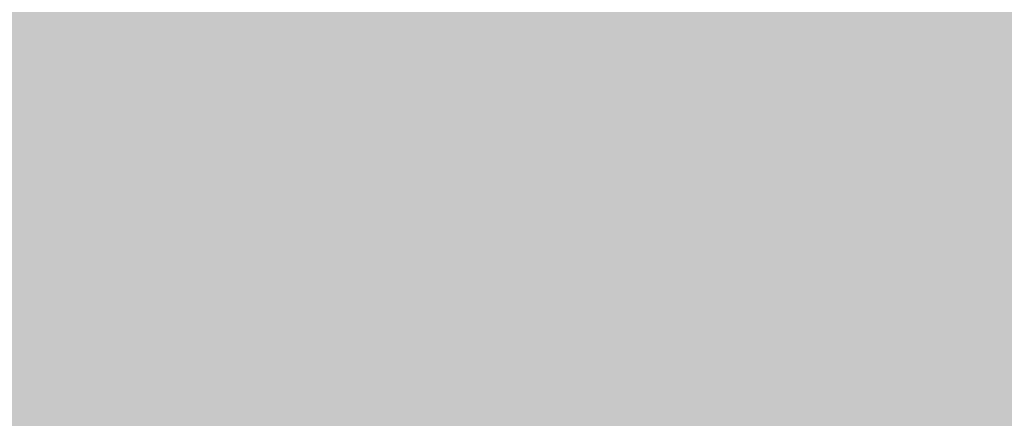
# Model space of a CAD drawing. Units: millimetres. Extents: x 0 to 2267, y 0 to 1823.
# Tile 130 of 256: x 1605.705 to 1611.042, y 1232.602 to 1234.764. Entities that reach past the tile are written whole.
import ezdxf

# ---------------------------------------------------------------- set-up
doc = ezdxf.new("R2010")
doc.units = ezdxf.units.MM
doc.header["$MEASUREMENT"] = 0
doc.layers.add('M-HATC', color=252, linetype='Continuous', lineweight=18)

msp = doc.modelspace()

# ---------------------------------------------------------------- hatches: boundary and pattern name
at = {"layer": 'M-HATC'}
h = msp.add_hatch(color=256, dxfattribs=at)
h.dxf.hatch_style = 1
h.paths.add_polyline_path([(2065.771, 1618.062, 0.236068), (2055.771, 1638.062), (1381.0868, 1638.062, 0.236068), (1371.0868, 1618.062), (1371.0868, 1603.062), (2055.771, 1603.062), (2065.771, 1603.062)])
h.paths.add_polyline_path([(2062.7718, 1550.2964), (2062.7718, 1560.2964), (1374.086, 1560.2964), (1374.086, 1550.2964), (1374.086, 1540.2964), (1384.086, 1540.2964), (1389.086, 1540.2964), (2062.7718, 1540.2964)])
h.paths.add_polyline_path([(1930.9289, 1282.7656), (1505.9289, 1282.7656), (1587.6276, 1235.5968, 0.131652), (1600.1276, 1232.2475), (1836.7302, 1232.2475, 0.131652), (1849.2302, 1235.5968)])
h.paths.add_polyline_path([(1930.9289, 1117.4171), (1905.9289, 1117.4171), (1505.9289, 1117.4171), (1505.9289, 1077.4171), (1930.9289, 1077.4171)])
h = msp.add_hatch(color=256, dxfattribs=at)
h.dxf.hatch_style = 1
h.paths.add_polyline_path([(2055.771, 1603.062), (1381.0868, 1603.062), (1381.0868, 1598.062), (2055.771, 1598.062)])
h.paths.add_polyline_path([(2055.771, 1598.062), (1381.0868, 1598.062), (1381.0868, 1593.062), (2055.771, 1593.062)])
h.paths.add_polyline_path([(2051.3074, 1536.7609), (1385.5504, 1536.7609), (1385.5504, 1526.7609), (1387.5504, 1526.7609), (1388.5366, 1525.0528), (1385.3319, 1521.2335), (1385.3319, 1521.2226), (2050.2542, 1522.7491), (2048.3212, 1525.0528), (2049.3074, 1526.7609), (2051.3074, 1526.7609)])
edge = h.paths.add_edge_path()
edge.add_arc((1847.5345, 1379.1492), 135, 222.603061, 222.890851, ccw=False)
edge.add_line((1748.1663, 1287.7656), (1683.0921, 1287.7656))
edge.add_arc((1583.7239, 1379.1492), 135, 317.109149, 317.396939, ccw=False)
edge.add_arc((1678.9686, 1290.6707), 5, 222.8909, 317.1091, ccw=False)
edge.add_arc((1774.2133, 1379.1492), 135, 222.603061, 222.890851, ccw=False)
edge.add_line((1674.8451, 1287.7656), (1609.7709, 1287.7656))
edge.add_arc((1510.4027, 1379.1492), 135, 317.109149, 317.396939, ccw=False)
edge.add_arc((1605.6474, 1290.6707), 5, 222.8909, 317.1091, ccw=False)
edge.add_arc((1700.8921, 1379.1492), 135, 222.603061, 222.890851, ccw=False)
edge.add_line((1601.5239, 1287.7656), (1536.4497, 1287.7656))
edge.add_arc((1437.0815, 1379.1492), 135, 317.109149, 317.396939, ccw=False)
edge.add_arc((1532.3262, 1290.6707), 5, 222.8909, 317.1091, ccw=False)
edge.add_arc((1627.5709, 1379.1492), 135, 222.603061, 222.890851, ccw=False)
edge.add_line((1528.2027, 1287.7656), (1505.9289, 1287.7656))
edge.add_spline(control_points=[(1505.9289, 1287.7656), (1504.2622, 1287.7656), (1504.2622, 1282.7656), (1505.9289, 1282.7656)], knot_values=[0, 0, 0, 0, 5, 5, 5, 5], degree=3, periodic=0)
edge.add_line((1505.9289, 1282.7656), (1930.9289, 1282.7656))
edge.add_spline(control_points=[(1930.9289, 1282.7656), (1932.5956, 1282.7656), (1932.5956, 1287.7656), (1930.9289, 1287.7656)], knot_values=[0, 0, 0, 0, 5, 5, 5, 5], degree=3, periodic=0)
edge.add_line((1930.9289, 1287.7656), (1903.0557, 1287.7656))
edge.add_arc((1803.6875, 1379.1492), 135, 317.109149, 317.396939, ccw=False)
edge.add_arc((1898.9322, 1290.6707), 5, 222.8909, 317.1091, ccw=False)
edge.add_arc((1994.1769, 1379.1492), 135, 222.603061, 222.890851, ccw=False)
edge.add_line((1894.8087, 1287.7656), (1829.7345, 1287.7656))
edge.add_arc((1730.3663, 1379.1492), 135, 317.109149, 317.396939, ccw=False)
edge.add_arc((1825.611, 1290.6707), 5, 222.8909, 317.1091, ccw=False)
edge.add_arc((1920.8557, 1379.1492), 135, 222.603061, 222.890851, ccw=False)
edge.add_line((1821.4875, 1287.7656), (1756.4133, 1287.7656))
edge.add_arc((1657.0451, 1379.1492), 135, 317.109149, 317.396939, ccw=False)
edge.add_arc((1752.2898, 1290.6707), 5, 222.8909, 317.1091, ccw=False)
edge = h.paths.add_edge_path()
edge.add_spline(control_points=[(1843.4289, 1227.2475), (1845.0956, 1227.2475), (1845.0956, 1232.2475), (1843.4289, 1232.2475)], knot_values=[0, 0, 0, 0, 5, 5, 5, 5], degree=3, periodic=0)
edge.add_line((1843.4289, 1232.2475), (1593.4289, 1232.2475))
edge.add_spline(control_points=[(1593.4289, 1232.2475), (1591.7622, 1232.2475), (1591.7622, 1227.2475), (1593.4289, 1227.2475)], knot_values=[0, 0, 0, 0, 5, 5, 5, 5], degree=3, periodic=0)
edge.add_line((1593.4289, 1227.2475), (1843.4289, 1227.2475))
h.paths.add_polyline_path([(1905.9289, 1127.4171), (1530.9289, 1127.4171, 0.414214), (1520.9289, 1117.4171), (1530.9289, 1117.4171), (1915.9289, 1117.4171, 0.414214)])
edge = h.paths.add_edge_path()
edge.add_arc((1397.0858, 1498.4078), 12.7299, 90.78215, 190.87871, ccw=False)
edge.add_line((1396.912, 1511.1365), (1428.0097, 1511.3488))
edge.add_line((1428.0097, 1511.3488), (1433.0097, 1511.3488))
edge.add_line((1433.0097, 1511.3488), (1434.439, 1511.3488))
edge.add_arc((1419.474, 1498.0804), 20, 41.561, 74.08211)
edge.add_line((1424.9592, 1517.3135), (1399.9351, 1517.2561))
edge.add_spline(control_points=[(1399.9307, 1517.2561), (1399.884, 1517.2131), (1399.8328, 1517.1689), (1399.7774, 1517.1236)], knot_values=[11.567499, 11.567499, 11.567499, 11.567499, 11.814249, 11.814249, 11.814249, 11.814249], degree=3, periodic=0)
edge.add_spline(control_points=[(1399.6328, 1517.0099), (1399.5831, 1516.9721), (1399.5307, 1516.9338), (1399.4759, 1516.8947)], knot_values=[11.167718, 11.167718, 11.167718, 11.167718, 11.365188, 11.365188, 11.365188, 11.365188], degree=3, periodic=0)
edge.add_spline(control_points=[(1399.3398, 1516.8001), (1399.1514, 1516.6719), (1398.9384, 1516.5377), (1398.704, 1516.3994)], knot_values=[10.376405, 10.376405, 10.376405, 10.376405, 11.00994, 11.00994, 11.00994, 11.00994], degree=3, periodic=0)
edge.add_spline(control_points=[(1398.6572, 1516.3719), (1398.5789, 1516.326), (1398.4983, 1516.2797), (1398.4155, 1516.2331)], knot_values=[10.125175, 10.125175, 10.125175, 10.125175, 10.334406, 10.334406, 10.334406, 10.334406], degree=3, periodic=0)
edge.add_spline(control_points=[(1398.2642, 1516.1487), (1398.196, 1516.1111), (1398.1263, 1516.0732), (1398.0555, 1516.0351)], knot_values=[9.832246, 9.832246, 9.832246, 9.832246, 9.999658, 9.999658, 9.999658, 9.999658], degree=3, periodic=0)
edge.add_spline(control_points=[(1397.9987, 1516.0048), (1397.7312, 1515.8621), (1397.446, 1515.7171), (1397.1466, 1515.5714)], knot_values=[9.161808, 9.161808, 9.161808, 9.161808, 9.787769, 9.787769, 9.787769, 9.787769], degree=3, periodic=0)
edge.add_spline(control_points=[(1397.1466, 1515.5714), (1396.8418, 1515.423), (1396.5222, 1515.274), (1396.1914, 1515.1262)], knot_values=[8.524455, 8.524455, 8.524455, 8.524455, 9.161808, 9.161808, 9.161808, 9.161808], degree=3, periodic=0)
edge.add_spline(control_points=[(1396.0777, 1515.0756), (1395.9854, 1515.0348), (1395.8922, 1514.994), (1395.7983, 1514.9534)], knot_values=[8.275193, 8.275193, 8.275193, 8.275193, 8.451726, 8.451726, 8.451726, 8.451726], degree=3, periodic=0)
edge.add_spline(control_points=[(1395.6018, 1514.8691), (1395.4997, 1514.8257), (1395.3968, 1514.7824), (1395.2932, 1514.7394)], knot_values=[7.962917, 7.962917, 7.962917, 7.962917, 8.152764, 8.152764, 8.152764, 8.152764], degree=3, periodic=0)
edge.add_spline(control_points=[(1395.2116, 1514.7057), (1394.8278, 1514.5475), (1394.4345, 1514.3929), (1394.0364, 1514.2442)], knot_values=[7.21254, 7.21254, 7.21254, 7.21254, 7.913148, 7.913148, 7.913148, 7.913148], degree=3, periodic=0)
edge.add_spline(control_points=[(1394.0364, 1514.2442), (1393.7076, 1514.1214), (1393.3754, 1514.0027), (1393.0427, 1513.8895)], knot_values=[6.633733, 6.633733, 6.633733, 6.633733, 7.21254, 7.21254, 7.21254, 7.21254], degree=3, periodic=0)
edge.add_spline(control_points=[(1392.8214, 1513.815), (1392.7198, 1513.7812), (1392.6181, 1513.7479), (1392.5166, 1513.7152)], knot_values=[6.328796, 6.328796, 6.328796, 6.328796, 6.505493, 6.505493, 6.505493, 6.505493], degree=3, periodic=0)
edge.add_spline(control_points=[(1392.5166, 1513.7152), (1392.3187, 1513.6515), (1392.1212, 1513.59), (1391.9244, 1513.531)], knot_values=[5.984605, 5.984605, 5.984605, 5.984605, 6.328796, 6.328796, 6.328796, 6.328796], degree=3, periodic=0)
edge.add_spline(control_points=[(1391.7915, 1513.4915), (1391.3122, 1513.3501), (1390.8384, 1513.2239), (1390.3784, 1513.1171)], knot_values=[5.066697, 5.066697, 5.066697, 5.066697, 5.907055, 5.907055, 5.907055, 5.907055], degree=3, periodic=0)
edge.add_spline(control_points=[(1390.3784, 1513.1171), (1390.1797, 1513.071), (1389.9836, 1513.0284), (1389.7907, 1512.9899)], knot_values=[4.70367, 4.70367, 4.70367, 4.70367, 5.066695, 5.066695, 5.066695, 5.066695], degree=3, periodic=0)
edge.add_spline(control_points=[(1389.422, 1512.9204), (1389.2459, 1512.8892), (1389.0729, 1512.8617), (1388.9036, 1512.8381)], knot_values=[4.130571, 4.130571, 4.130571, 4.130571, 4.469816, 4.469816, 4.469816, 4.469816], degree=3, periodic=0)
edge.add_spline(control_points=[(1388.9036, 1512.8381), (1388.591, 1512.7946), (1388.2911, 1512.7644), (1388.0071, 1512.7494)], knot_values=[3.504031, 3.504031, 3.504031, 3.504031, 4.130571, 4.130571, 4.130571, 4.130571], degree=3, periodic=0)
edge.add_spline(control_points=[(1387.9356, 1512.7459), (1387.8538, 1512.7423), (1387.7733, 1512.74), (1387.6944, 1512.739)], knot_values=[3.268866, 3.268866, 3.268866, 3.268866, 3.451164, 3.451164, 3.451164, 3.451164], degree=3, periodic=0)
edge.add_spline(control_points=[(1387.3351, 1512.7443), (1387.2076, 1512.7499), (1387.0847, 1512.7597), (1386.967, 1512.7739)], knot_values=[2.670686, 2.670686, 2.670686, 2.670686, 2.984, 2.984, 2.984, 2.984], degree=3, periodic=0)
edge.add_spline(control_points=[(1386.8327, 1512.7922), (1386.8209, 1512.7941), (1386.8092, 1512.7959), (1386.7975, 1512.7979)], knot_values=[2.516981, 2.516981, 2.516981, 2.516981, 2.549528, 2.549528, 2.549528, 2.549528], degree=3, periodic=0)
edge.add_spline(control_points=[(1386.4526, 1512.8735), (1386.4257, 1512.881), (1386.3993, 1512.889), (1386.3733, 1512.8972)], knot_values=[2.095869, 2.095869, 2.095869, 2.095869, 2.17941, 2.17941, 2.17941, 2.17941], degree=3, periodic=0)
edge.add_spline(control_points=[(1386.0691, 1513.0189), (1386.0634, 1513.0217), (1386.0577, 1513.0246), (1386.052, 1513.0275)], knot_values=[1.72453, 1.72453, 1.72453, 1.72453, 1.745933, 1.745933, 1.745933, 1.745933], degree=3, periodic=0)
edge.add_arc((1399.474, 1498.0804), 20, 131.82432, 180)
edge.add_arc((1630.3336, 1505.5484), 250.9708, 181.705176, 236.427975)
edge.add_arc((1605.3399, 1483.3044), 218.7822, 238.660829, 243.34961)
edge.add_arc((1647.0911, 1510.3592), 262.8986, 183.129836, 237.853442, ccw=False)
h.paths.add_polyline_path([(1406.5369, 1391.9644, 0.149382), (1491.5506, 1296.4418, -0.129517)], flags=17)
edge = h.paths.add_edge_path()
edge.add_arc((2037.3838, 1498.0804), 20, 0, 48.26587)
edge.add_spline(control_points=[(2050.6973, 1513.0052), (2050.6512, 1512.9847), (2050.6034, 1512.9655), (2050.5539, 1512.9477)], knot_values=[1.835652, 1.835652, 1.835652, 1.835652, 2.000781, 2.000781, 2.000781, 2.000781], degree=3, periodic=0)
edge.add_spline(control_points=[(2050.4616, 1512.9166), (2050.479, 1512.9221), (2050.4963, 1512.9277), (2050.5133, 1512.9335)], knot_values=[2.045477, 2.045477, 2.045477, 2.045477, 2.101389, 2.101389, 2.101389, 2.101389], degree=3, periodic=0)
edge.add_spline(control_points=[(2050.129, 1512.8342), (2050.1984, 1512.8473), (2050.2657, 1512.8623), (2050.3308, 1512.8792)], knot_values=[2.237629, 2.237629, 2.237629, 2.237629, 2.435841, 2.435841, 2.435841, 2.435841], degree=3, periodic=0)
edge.add_spline(control_points=[(2050.0946, 1512.8278), (2050.1061, 1512.8299), (2050.1176, 1512.832), (2050.129, 1512.8342)], knot_values=[2.435841, 2.435841, 2.435841, 2.435841, 2.468321, 2.468321, 2.468321, 2.468321], degree=3, periodic=0)
edge.add_spline(control_points=[(2049.7843, 1512.7851), (2049.8552, 1512.7922), (2049.9243, 1512.8008), (2049.9917, 1512.8109)], knot_values=[2.563852, 2.563852, 2.563852, 2.563852, 2.748541, 2.748541, 2.748541, 2.748541], degree=3, periodic=0)
edge.add_spline(control_points=[(2049.4052, 1512.7617), (2049.5364, 1512.7653), (2049.6629, 1512.773), (2049.7843, 1512.7851)], knot_values=[2.748541, 2.748541, 2.748541, 2.748541, 3.064882, 3.064882, 3.064882, 3.064882], degree=3, periodic=0)
edge.add_spline(control_points=[(2049.1698, 1512.7597), (2049.2336, 1512.7591), (2049.2965, 1512.7594), (2049.3584, 1512.7606)], knot_values=[3.102309, 3.102309, 3.102309, 3.102309, 3.2503, 3.2503, 3.2503, 3.2503], degree=3, periodic=0)
edge.add_spline(control_points=[(2048.8573, 1512.7691), (2048.9638, 1512.7638), (2049.068, 1512.7606), (2049.1698, 1512.7597)], knot_values=[3.2503, 3.2503, 3.2503, 3.2503, 3.486069, 3.486069, 3.486069, 3.486069], degree=3, periodic=0)
edge.add_spline(control_points=[(2048.6924, 1512.7789), (2048.3729, 1512.8009), (2048.0345, 1512.8411), (2047.6817, 1512.897)], knot_values=[3.606429, 3.606429, 3.606429, 3.606429, 4.2989, 4.2989, 4.2989, 4.2989], degree=3, periodic=0)
edge.add_spline(control_points=[(2047.6817, 1512.897), (2047.5458, 1512.9185), (2047.4077, 1512.9424), (2047.2678, 1512.9685)], knot_values=[4.2989, 4.2989, 4.2989, 4.2989, 4.565769, 4.565769, 4.565769, 4.565769], degree=3, periodic=0)
edge.add_spline(control_points=[(2047.2678, 1512.9685), (2047.1449, 1512.9914), (2047.0207, 1513.016), (2046.8951, 1513.0422)], knot_values=[4.565769, 4.565769, 4.565769, 4.565769, 4.799971, 4.799971, 4.799971, 4.799971], degree=3, periodic=0)
edge.add_spline(control_points=[(2046.8951, 1513.0422), (2046.5286, 1513.1188), (2046.1513, 1513.209), (2045.7676, 1513.3107)], knot_values=[4.799971, 4.799971, 4.799971, 4.799971, 5.483718, 5.483718, 5.483718, 5.483718], degree=3, periodic=0)
edge.add_spline(control_points=[(2045.7676, 1513.3107), (2045.3724, 1513.4154), (2044.9704, 1513.5322), (2044.5662, 1513.6588)], knot_values=[5.483718, 5.483718, 5.483718, 5.483718, 6.187866, 6.187866, 6.187866, 6.187866], degree=3, periodic=0)
edge.add_spline(control_points=[(2044.5662, 1513.6588), (2044.4149, 1513.7061), (2044.2633, 1513.7549), (2044.1116, 1513.8048)], knot_values=[6.187866, 6.187866, 6.187866, 6.187866, 6.451551, 6.451551, 6.451551, 6.451551], degree=3, periodic=0)
edge.add_spline(control_points=[(2044.1116, 1513.8048), (2043.9967, 1513.8427), (2043.8817, 1513.8813), (2043.7668, 1513.9205)], knot_values=[6.451551, 6.451551, 6.451551, 6.451551, 6.651434, 6.651434, 6.651434, 6.651434], degree=3, periodic=0)
edge.add_spline(control_points=[(2043.7668, 1513.9205), (2043.3716, 1514.0554), (2042.9774, 1514.1979), (2042.5886, 1514.3458)], knot_values=[6.651434, 6.651434, 6.651434, 6.651434, 7.338879, 7.338879, 7.338879, 7.338879], degree=3, periodic=0)
edge.add_spline(control_points=[(2042.5886, 1514.3458), (2042.1643, 1514.5071), (2041.7465, 1514.6749), (2041.3409, 1514.846)], knot_values=[7.338879, 7.338879, 7.338879, 7.338879, 8.089209, 8.089209, 8.089209, 8.089209], degree=3, periodic=0)
edge.add_spline(control_points=[(2041.3409, 1514.846), (2041.1028, 1514.9465), (2040.869, 1515.0481), (2040.6405, 1515.1502)], knot_values=[8.089209, 8.089209, 8.089209, 8.089209, 8.529587, 8.529587, 8.529587, 8.529587], degree=3, periodic=0)
edge.add_spline(control_points=[(2040.51, 1515.2089), (2040.0824, 1515.4022), (2039.6747, 1515.5971), (2039.295, 1515.7894)], knot_values=[8.613818, 8.613818, 8.613818, 8.613818, 9.44571, 9.44571, 9.44571, 9.44571], degree=3, periodic=0)
edge.add_spline(control_points=[(2039.295, 1515.7894), (2039.0618, 1515.9075), (2038.8391, 1516.0246), (2038.6288, 1516.1398)], knot_values=[9.44571, 9.44571, 9.44571, 9.44571, 9.956404, 9.956404, 9.956404, 9.956404], degree=3, periodic=0)
edge.add_spline(control_points=[(2038.6288, 1516.1398), (2038.5187, 1516.2001), (2038.4121, 1516.2598), (2038.309, 1516.3189)], knot_values=[9.956404, 9.956404, 9.956404, 9.956404, 10.223542, 10.223542, 10.223542, 10.223542], degree=3, periodic=0)
edge.add_spline(control_points=[(2038.309, 1516.3189), (2038.2138, 1516.3735), (2038.1216, 1516.4276), (2038.0328, 1516.481)], knot_values=[10.223542, 10.223542, 10.223542, 10.223542, 10.47051, 10.47051, 10.47051, 10.47051], degree=3, periodic=0)
edge.add_spline(control_points=[(2038.0328, 1516.481), (2037.7855, 1516.6296), (2037.5639, 1516.773), (2037.3722, 1516.909)], knot_values=[10.47051, 10.47051, 10.47051, 10.47051, 11.15767, 11.15767, 11.15767, 11.15767], degree=3, periodic=0)
edge.add_spline(control_points=[(2037.3722, 1516.909), (2037.2789, 1516.9752), (2037.1927, 1517.0396), (2037.1142, 1517.102)], knot_values=[11.15767, 11.15767, 11.15767, 11.15767, 11.49227, 11.49227, 11.49227, 11.49227], degree=3, periodic=0)
edge.add_spline(control_points=[(2036.8564, 1517.3259), (2036.9148, 1517.2692), (2036.9814, 1517.2103), (2037.0557, 1517.1492)], knot_values=[11.577341, 11.577341, 11.577341, 11.577341, 11.91035, 11.91035, 11.91035, 11.91035], degree=3, periodic=0)
edge.add_spline(control_points=[(2036.8074, 1517.3748), (2036.823, 1517.3587), (2036.8393, 1517.3424), (2036.8564, 1517.3259)], knot_values=[11.91035, 11.91035, 11.91035, 11.91035, 12.007402, 12.007402, 12.007402, 12.007402], degree=3, periodic=0)
edge.add_spline(control_points=[(2036.7017, 1517.494), (2036.7104, 1517.483), (2036.7196, 1517.4719), (2036.7291, 1517.4606)], knot_values=[12.184155, 12.184155, 12.184155, 12.184155, 12.255409, 12.255409, 12.255409, 12.255409], degree=3, periodic=0)
edge.add_spline(control_points=[(2036.6159, 1517.6205), (2036.62, 1517.613), (2036.6243, 1517.6055), (2036.6289, 1517.5979)], knot_values=[12.487913, 12.487913, 12.487913, 12.487913, 12.541035, 12.541035, 12.541035, 12.541035], degree=3, periodic=0)
edge.add_spline(control_points=[(2036.5635, 1517.786), (2036.5637, 1517.7794), (2036.5642, 1517.7726), (2036.565, 1517.7658)], knot_values=[12.911761, 12.911761, 12.911761, 12.911761, 12.968286, 12.968286, 12.968286, 12.968286], degree=3, periodic=0)
edge.add_spline(control_points=[(2036.6166, 1517.9304), (2036.6125, 1517.9259), (2036.6086, 1517.9212), (2036.6049, 1517.9165)], knot_values=[13.382527, 13.382527, 13.382527, 13.382527, 13.433791, 13.433791, 13.433791, 13.433791], degree=3, periodic=0)
edge.add_spline(control_points=[(2036.749, 1518.017), (2036.7361, 1518.0116), (2036.7239, 1518.006), (2036.7124, 1518.0002)], knot_values=[13.726299, 13.726299, 13.726299, 13.726299, 13.809928, 13.809928, 13.809928, 13.809928], degree=3, periodic=0)
edge.add_spline(control_points=[(2036.8604, 1518.0528), (2036.8386, 1518.0474), (2036.8181, 1518.0416), (2036.7988, 1518.0353)], knot_values=[13.910887, 13.910887, 13.910887, 13.910887, 14.02153, 14.02153, 14.02153, 14.02153], degree=3, periodic=0)
edge.add_line((2036.9639, 1518.0804), (2032.3838, 1518.0804))
edge.add_line((2032.3838, 1518.0804), (2027.3838, 1518.0804))
edge.add_line((2027.3838, 1518.0804), (2022.3838, 1518.0804))
edge.add_line((2022.3838, 1518.0804), (2017.3838, 1518.0804))
edge.add_arc((2017.3838, 1498.0804), 20, 90, 138.439)
edge.add_line((2002.4188, 1511.3488), (2003.8481, 1511.3488))
edge.add_line((2003.8481, 1511.3488), (2008.8481, 1511.3488))
edge.add_line((2008.8481, 1511.3488), (2039.772, 1511.1377))
edge.add_arc((2039.772, 1498.4078), 12.7299, -10.87871, 90, ccw=False)
edge.add_arc((1789.7668, 1510.3592), 262.8986, 302.146558, 356.870164, ccw=False)
edge.add_arc((1831.5179, 1483.3044), 218.7822, 296.65039, 301.339171)
edge.add_arc((1806.5242, 1505.5484), 250.9708, 303.572025, 358.294824)
h.paths.add_polyline_path([(2030.321, 1391.9644, -0.129517), (1945.3072, 1296.4418, 0.149382)], flags=17)
edge = h.paths.add_edge_path()
edge.add_spline(control_points=[(2037.2464, 1518.0821), (2037.2898, 1518.081), (2037.3355, 1518.0804), (2037.3838, 1518.0804)], knot_values=[0.000012, 0.000012, 0.000012, 0.000012, 0.144754, 0.144754, 0.144754, 0.144754], degree=3, periodic=0)
edge.add_line((2037.3357, 1518.0804), (2037.0096, 1518.0804))
edge.add_spline(control_points=[(2037.0096, 1518.0804), (2036.9822, 1518.0768), (2036.956, 1518.0727), (2036.9312, 1518.0681)], knot_values=[14.13465, 14.13465, 14.13465, 14.13465, 14.247197, 14.247197, 14.247197, 14.247197], degree=3, periodic=0)
edge.add_spline(control_points=[(2036.9312, 1518.0681), (2036.9276, 1518.0674), (2036.9241, 1518.0667), (2036.9205, 1518.0661)], knot_values=[14.118315, 14.118315, 14.118315, 14.118315, 14.13465, 14.13465, 14.13465, 14.13465], degree=3, periodic=0)
edge.add_spline(control_points=[(2036.9205, 1518.0661), (2036.9118, 1518.0644), (2036.9032, 1518.0626), (2036.8948, 1518.0608)], knot_values=[14.078086, 14.078086, 14.078086, 14.078086, 14.118315, 14.118315, 14.118315, 14.118315], degree=3, periodic=0)
edge.add_spline(control_points=[(2036.8948, 1518.0608), (2036.883, 1518.0583), (2036.8716, 1518.0556), (2036.8604, 1518.0528)], knot_values=[14.02153, 14.02153, 14.02153, 14.02153, 14.078086, 14.078086, 14.078086, 14.078086], degree=3, periodic=0)
edge.add_spline(control_points=[(2036.8604, 1518.0528), (2036.8386, 1518.0474), (2036.8181, 1518.0416), (2036.7988, 1518.0353)], knot_values=[13.910887, 13.910887, 13.910887, 13.910887, 14.02153, 14.02153, 14.02153, 14.02153], degree=3, periodic=0)
edge.add_spline(control_points=[(2036.7988, 1518.0353), (2036.7981, 1518.035), (2036.7974, 1518.0348), (2036.7967, 1518.0346)], knot_values=[13.906906, 13.906906, 13.906906, 13.906906, 13.910887, 13.910887, 13.910887, 13.910887], degree=3, periodic=0)
edge.add_spline(control_points=[(2036.7967, 1518.0346), (2036.7882, 1518.0318), (2036.7799, 1518.0289), (2036.7719, 1518.0259)], knot_values=[13.857826, 13.857826, 13.857826, 13.857826, 13.906906, 13.906906, 13.906906, 13.906906], degree=3, periodic=0)
edge.add_spline(control_points=[(2036.7719, 1518.0259), (2036.764, 1518.023), (2036.7564, 1518.02), (2036.749, 1518.017)], knot_values=[13.809928, 13.809928, 13.809928, 13.809928, 13.857826, 13.857826, 13.857826, 13.857826], degree=3, periodic=0)
edge.add_spline(control_points=[(2036.749, 1518.017), (2036.7361, 1518.0116), (2036.7239, 1518.006), (2036.7124, 1518.0002)], knot_values=[13.726299, 13.726299, 13.726299, 13.726299, 13.809928, 13.809928, 13.809928, 13.809928], degree=3, periodic=0)
edge.add_spline(control_points=[(2036.7124, 1518.0002), (2036.7121, 1518), (2036.7118, 1517.9999), (2036.7115, 1517.9997)], knot_values=[13.723993, 13.723993, 13.723993, 13.723993, 13.726299, 13.726299, 13.726299, 13.726299], degree=3, periodic=0)
edge.add_spline(control_points=[(2036.7115, 1517.9997), (2036.7063, 1517.9971), (2036.7013, 1517.9944), (2036.6965, 1517.9917)], knot_values=[13.686536, 13.686536, 13.686536, 13.686536, 13.723993, 13.723993, 13.723993, 13.723993], degree=3, periodic=0)
edge.add_spline(control_points=[(2036.6965, 1517.9917), (2036.6919, 1517.9891), (2036.6874, 1517.9865), (2036.6831, 1517.9839)], knot_values=[13.651251, 13.651251, 13.651251, 13.651251, 13.686536, 13.686536, 13.686536, 13.686536], degree=3, periodic=0)
edge.add_spline(control_points=[(2036.6831, 1517.9839), (2036.6764, 1517.9798), (2036.67, 1517.9757), (2036.6639, 1517.9714)], knot_values=[13.596804, 13.596804, 13.596804, 13.596804, 13.651251, 13.651251, 13.651251, 13.651251], degree=3, periodic=0)
edge.add_spline(control_points=[(2036.6639, 1517.9714), (2036.6636, 1517.9712), (2036.6633, 1517.9709), (2036.6629, 1517.9707)], knot_values=[13.593956, 13.593956, 13.593956, 13.593956, 13.596804, 13.596804, 13.596804, 13.596804], degree=3, periodic=0)
edge.add_spline(control_points=[(2036.6629, 1517.9707), (2036.6603, 1517.9689), (2036.6577, 1517.967), (2036.6552, 1517.9651)], knot_values=[13.570322, 13.570322, 13.570322, 13.570322, 13.593956, 13.593956, 13.593956, 13.593956], degree=3, periodic=0)
edge.add_spline(control_points=[(2036.6552, 1517.9651), (2036.6525, 1517.9631), (2036.6499, 1517.9611), (2036.6474, 1517.9591)], knot_values=[13.545477, 13.545477, 13.545477, 13.545477, 13.570322, 13.570322, 13.570322, 13.570322], degree=3, periodic=0)
edge.add_spline(control_points=[(2036.6474, 1517.9591), (2036.6472, 1517.9589), (2036.6471, 1517.9588), (2036.6469, 1517.9587)], knot_values=[13.543931, 13.543931, 13.543931, 13.543931, 13.545477, 13.545477, 13.545477, 13.545477], degree=3, periodic=0)
edge.add_spline(control_points=[(2036.6469, 1517.9587), (2036.6412, 1517.9541), (2036.6358, 1517.9494), (2036.6307, 1517.9447)], knot_values=[13.488237, 13.488237, 13.488237, 13.488237, 13.543931, 13.543931, 13.543931, 13.543931], degree=3, periodic=0)
edge.add_spline(control_points=[(2036.6307, 1517.9447), (2036.6282, 1517.9423), (2036.6257, 1517.9399), (2036.6233, 1517.9374)], knot_values=[13.460307, 13.460307, 13.460307, 13.460307, 13.488237, 13.488237, 13.488237, 13.488237], degree=3, periodic=0)
edge.add_spline(control_points=[(2036.6233, 1517.9374), (2036.6215, 1517.9356), (2036.6198, 1517.9338), (2036.6181, 1517.932)], knot_values=[13.439712, 13.439712, 13.439712, 13.439712, 13.460307, 13.460307, 13.460307, 13.460307], degree=3, periodic=0)
edge.add_spline(control_points=[(2036.6181, 1517.932), (2036.6176, 1517.9315), (2036.6171, 1517.9309), (2036.6166, 1517.9304)], knot_values=[13.433791, 13.433791, 13.433791, 13.433791, 13.439712, 13.439712, 13.439712, 13.439712], degree=3, periodic=0)
edge.add_spline(control_points=[(2036.6166, 1517.9304), (2036.6125, 1517.9259), (2036.6086, 1517.9212), (2036.6049, 1517.9165)], knot_values=[13.382527, 13.382527, 13.382527, 13.382527, 13.433791, 13.433791, 13.433791, 13.433791], degree=3, periodic=0)
edge.add_spline(control_points=[(2036.6049, 1517.9165), (2036.6026, 1517.9135), (2036.6004, 1517.9104), (2036.5982, 1517.9074)], knot_values=[13.350017, 13.350017, 13.350017, 13.350017, 13.382527, 13.382527, 13.382527, 13.382527], degree=3, periodic=0)
edge.add_spline(control_points=[(2036.5982, 1517.9074), (2036.5972, 1517.9059), (2036.5962, 1517.9043), (2036.5952, 1517.9028)], knot_values=[13.333922, 13.333922, 13.333922, 13.333922, 13.350017, 13.350017, 13.350017, 13.350017], degree=3, periodic=0)
edge.add_spline(control_points=[(2036.5952, 1517.9028), (2036.5945, 1517.9018), (2036.5939, 1517.9009), (2036.5933, 1517.8999)], knot_values=[13.323828, 13.323828, 13.323828, 13.323828, 13.333922, 13.333922, 13.333922, 13.333922], degree=3, periodic=0)
edge.add_spline(control_points=[(2036.5933, 1517.8999), (2036.5905, 1517.8955), (2036.5879, 1517.8909), (2036.5855, 1517.8864)], knot_values=[13.277545, 13.277545, 13.277545, 13.277545, 13.323828, 13.323828, 13.323828, 13.323828], degree=3, periodic=0)
edge.add_spline(control_points=[(2036.5855, 1517.8864), (2036.5836, 1517.8827), (2036.5817, 1517.8789), (2036.5801, 1517.8751)], knot_values=[13.240119, 13.240119, 13.240119, 13.240119, 13.277545, 13.277545, 13.277545, 13.277545], degree=3, periodic=0)
edge.add_spline(control_points=[(2036.5801, 1517.8751), (2036.5795, 1517.8739), (2036.579, 1517.8727), (2036.5785, 1517.8715)], knot_values=[13.228211, 13.228211, 13.228211, 13.228211, 13.240119, 13.240119, 13.240119, 13.240119], degree=3, periodic=0)
edge.add_spline(control_points=[(2036.5785, 1517.8715), (2036.578, 1517.8702), (2036.5774, 1517.869), (2036.5769, 1517.8677)], knot_values=[13.215717, 13.215717, 13.215717, 13.215717, 13.228211, 13.228211, 13.228211, 13.228211], degree=3, periodic=0)
edge.add_spline(control_points=[(2036.5769, 1517.8677), (2036.5755, 1517.864), (2036.5741, 1517.8603), (2036.5729, 1517.8565)], knot_values=[13.179847, 13.179847, 13.179847, 13.179847, 13.215717, 13.215717, 13.215717, 13.215717], degree=3, periodic=0)
edge.add_spline(control_points=[(2036.5729, 1517.8565), (2036.5713, 1517.8515), (2036.5699, 1517.8464), (2036.5687, 1517.8413)], knot_values=[13.132017, 13.132017, 13.132017, 13.132017, 13.179847, 13.179847, 13.179847, 13.179847], degree=3, periodic=0)
edge.add_spline(control_points=[(2036.5687, 1517.8413), (2036.5684, 1517.8402), (2036.5682, 1517.8392), (2036.568, 1517.8382)], knot_values=[13.122482, 13.122482, 13.122482, 13.122482, 13.132017, 13.132017, 13.132017, 13.132017], degree=3, periodic=0)
edge.add_spline(control_points=[(2036.568, 1517.8382), (2036.5676, 1517.8363), (2036.5672, 1517.8345), (2036.5669, 1517.8327)], knot_values=[13.105592, 13.105592, 13.105592, 13.105592, 13.122482, 13.122482, 13.122482, 13.122482], degree=3, periodic=0)
edge.add_spline(control_points=[(2036.5669, 1517.8327), (2036.5662, 1517.8292), (2036.5657, 1517.8257), (2036.5652, 1517.8222)], knot_values=[13.074063, 13.074063, 13.074063, 13.074063, 13.105592, 13.105592, 13.105592, 13.105592], degree=3, periodic=0)
edge.add_spline(control_points=[(2036.5652, 1517.8222), (2036.5652, 1517.8222), (2036.5652, 1517.8222), (2036.5652, 1517.8222)], knot_values=[13.074043, 13.074043, 13.074043, 13.074043, 13.074063, 13.074063, 13.074063, 13.074063], degree=3, periodic=0)
edge.add_spline(control_points=[(2036.5652, 1517.8222), (2036.5644, 1517.8164), (2036.5639, 1517.8106), (2036.5636, 1517.8046)], knot_values=[13.021884, 13.021884, 13.021884, 13.021884, 13.074043, 13.074043, 13.074043, 13.074043], degree=3, periodic=0)
edge.add_spline(control_points=[(2036.5636, 1517.8046), (2036.5636, 1517.804), (2036.5636, 1517.8034), (2036.5635, 1517.8028)], knot_values=[13.01674, 13.01674, 13.01674, 13.01674, 13.021884, 13.021884, 13.021884, 13.021884], degree=3, periodic=0)
edge.add_spline(control_points=[(2036.5635, 1517.8028), (2036.5634, 1517.8005), (2036.5634, 1517.7982), (2036.5634, 1517.7958)], knot_values=[12.996438, 12.996438, 12.996438, 12.996438, 13.01674, 13.01674, 13.01674, 13.01674], degree=3, periodic=0)
edge.add_spline(control_points=[(2036.5634, 1517.7958), (2036.5633, 1517.7926), (2036.5634, 1517.7893), (2036.5635, 1517.786)], knot_values=[12.968286, 12.968286, 12.968286, 12.968286, 12.996438, 12.996438, 12.996438, 12.996438], degree=3, periodic=0)
edge.add_spline(control_points=[(2036.5635, 1517.786), (2036.5637, 1517.7794), (2036.5642, 1517.7726), (2036.565, 1517.7658)], knot_values=[12.911761, 12.911761, 12.911761, 12.911761, 12.968286, 12.968286, 12.968286, 12.968286], degree=3, periodic=0)
edge.add_spline(control_points=[(2036.565, 1517.7658), (2036.565, 1517.7657), (2036.565, 1517.7656), (2036.565, 1517.7656)], knot_values=[12.911017, 12.911017, 12.911017, 12.911017, 12.911761, 12.911761, 12.911761, 12.911761], degree=3, periodic=0)
edge.add_spline(control_points=[(2036.565, 1517.7656), (2036.5654, 1517.7625), (2036.5658, 1517.7593), (2036.5663, 1517.7562)], knot_values=[12.88528, 12.88528, 12.88528, 12.88528, 12.911017, 12.911017, 12.911017, 12.911017], degree=3, periodic=0)
edge.add_spline(control_points=[(2036.5663, 1517.7562), (2036.5667, 1517.7534), (2036.5672, 1517.7506), (2036.5677, 1517.7478)], knot_values=[12.862519, 12.862519, 12.862519, 12.862519, 12.88528, 12.88528, 12.88528, 12.88528], degree=3, periodic=0)
edge.add_spline(control_points=[(2036.5677, 1517.7478), (2036.5678, 1517.7474), (2036.5679, 1517.7469), (2036.568, 1517.7465)], knot_values=[12.858885, 12.858885, 12.858885, 12.858885, 12.862519, 12.862519, 12.862519, 12.862519], degree=3, periodic=0)
edge.add_spline(control_points=[(2036.568, 1517.7465), (2036.5692, 1517.7399), (2036.5707, 1517.7332), (2036.5724, 1517.7264)], knot_values=[12.8053, 12.8053, 12.8053, 12.8053, 12.858885, 12.858885, 12.858885, 12.858885], degree=3, periodic=0)
edge.add_spline(control_points=[(2036.5724, 1517.7264), (2036.5734, 1517.7226), (2036.5745, 1517.7187), (2036.5756, 1517.7149)], knot_values=[12.775176, 12.775176, 12.775176, 12.775176, 12.8053, 12.8053, 12.8053, 12.8053], degree=3, periodic=0)
edge.add_spline(control_points=[(2036.5756, 1517.7149), (2036.5763, 1517.7125), (2036.577, 1517.7102), (2036.5778, 1517.7078)], knot_values=[12.756759, 12.756759, 12.756759, 12.756759, 12.775176, 12.775176, 12.775176, 12.775176], degree=3, periodic=0)
edge.add_spline(control_points=[(2036.5778, 1517.7078), (2036.5781, 1517.7067), (2036.5784, 1517.7057), (2036.5787, 1517.7047)], knot_values=[12.748742, 12.748742, 12.748742, 12.748742, 12.756759, 12.756759, 12.756759, 12.756759], degree=3, periodic=0)
edge.add_spline(control_points=[(2036.5787, 1517.7047), (2036.5808, 1517.6983), (2036.5831, 1517.6919), (2036.5856, 1517.6854)], knot_values=[12.69959, 12.69959, 12.69959, 12.69959, 12.748742, 12.748742, 12.748742, 12.748742], degree=3, periodic=0)
edge.add_spline(control_points=[(2036.5856, 1517.6854), (2036.5876, 1517.68), (2036.5898, 1517.6746), (2036.5921, 1517.6692)], knot_values=[12.659038, 12.659038, 12.659038, 12.659038, 12.69959, 12.69959, 12.69959, 12.69959], degree=3, periodic=0)
edge.add_spline(control_points=[(2036.5921, 1517.6692), (2036.594, 1517.6648), (2036.5959, 1517.6605), (2036.5979, 1517.6561)], knot_values=[12.626806, 12.626806, 12.626806, 12.626806, 12.659038, 12.659038, 12.659038, 12.659038], degree=3, periodic=0)
edge.add_spline(control_points=[(2036.5979, 1517.6561), (2036.5984, 1517.6551), (2036.5989, 1517.6541), (2036.5993, 1517.6531)], knot_values=[12.619394, 12.619394, 12.619394, 12.619394, 12.626806, 12.626806, 12.626806, 12.626806], degree=3, periodic=0)
edge.add_spline(control_points=[(2036.5993, 1517.6531), (2036.6043, 1517.6424), (2036.6099, 1517.6315), (2036.6159, 1517.6205)], knot_values=[12.541039, 12.541039, 12.541039, 12.541039, 12.619394, 12.619394, 12.619394, 12.619394], degree=3, periodic=0)
edge.add_spline(control_points=[(2036.6159, 1517.6205), (2036.6159, 1517.6205), (2036.6159, 1517.6205), (2036.6159, 1517.6205)], knot_values=[12.541035, 12.541035, 12.541035, 12.541035, 12.541039, 12.541039, 12.541039, 12.541039], degree=3, periodic=0)
edge.add_spline(control_points=[(2036.6159, 1517.6205), (2036.62, 1517.613), (2036.6243, 1517.6055), (2036.6289, 1517.5979)], knot_values=[12.487913, 12.487913, 12.487913, 12.487913, 12.541035, 12.541035, 12.541035, 12.541035], degree=3, periodic=0)
edge.add_spline(control_points=[(2036.6289, 1517.5979), (2036.6326, 1517.5916), (2036.6365, 1517.5853), (2036.6406, 1517.5789)], knot_values=[12.443982, 12.443982, 12.443982, 12.443982, 12.487913, 12.487913, 12.487913, 12.487913], degree=3, periodic=0)
edge.add_spline(control_points=[(2036.6406, 1517.5789), (2036.6414, 1517.5776), (2036.6423, 1517.5763), (2036.6431, 1517.5749)], knot_values=[12.434996, 12.434996, 12.434996, 12.434996, 12.443982, 12.443982, 12.443982, 12.443982], degree=3, periodic=0)
edge.add_spline(control_points=[(2036.6431, 1517.5749), (2036.6531, 1517.5596), (2036.6639, 1517.5439), (2036.6756, 1517.528)], knot_values=[12.329647, 12.329647, 12.329647, 12.329647, 12.434996, 12.434996, 12.434996, 12.434996], degree=3, periodic=0)
edge.add_spline(control_points=[(2036.6756, 1517.528), (2036.6839, 1517.5168), (2036.6925, 1517.5055), (2036.7017, 1517.494)], knot_values=[12.255409, 12.255409, 12.255409, 12.255409, 12.329647, 12.329647, 12.329647, 12.329647], degree=3, periodic=0)
edge.add_spline(control_points=[(2036.7017, 1517.494), (2036.7104, 1517.483), (2036.7196, 1517.4719), (2036.7291, 1517.4606)], knot_values=[12.184155, 12.184155, 12.184155, 12.184155, 12.255409, 12.255409, 12.255409, 12.255409], degree=3, periodic=0)
edge.add_spline(control_points=[(2036.7291, 1517.4606), (2036.7436, 1517.4435), (2036.759, 1517.4262), (2036.7753, 1517.4085)], knot_values=[12.075961, 12.075961, 12.075961, 12.075961, 12.184155, 12.184155, 12.184155, 12.184155], degree=3, periodic=0)
edge.add_spline(control_points=[(2036.7753, 1517.4085), (2036.7763, 1517.4075), (2036.7773, 1517.4064), (2036.7783, 1517.4054)], knot_values=[12.069502, 12.069502, 12.069502, 12.069502, 12.075961, 12.075961, 12.075961, 12.075961], degree=3, periodic=0)
edge.add_spline(control_points=[(2036.7783, 1517.4054), (2036.7877, 1517.3953), (2036.7974, 1517.385), (2036.8074, 1517.3748)], knot_values=[12.007402, 12.007402, 12.007402, 12.007402, 12.069502, 12.069502, 12.069502, 12.069502], degree=3, periodic=0)
edge.add_spline(control_points=[(2036.8074, 1517.3748), (2036.823, 1517.3587), (2036.8393, 1517.3424), (2036.8564, 1517.3259)], knot_values=[11.91035, 11.91035, 11.91035, 11.91035, 12.007402, 12.007402, 12.007402, 12.007402], degree=3, periodic=0)
edge.add_spline(control_points=[(2036.8564, 1517.3259), (2036.9148, 1517.2692), (2036.9814, 1517.2103), (2037.0557, 1517.1492)], knot_values=[11.577341, 11.577341, 11.577341, 11.577341, 11.91035, 11.91035, 11.91035, 11.91035], degree=3, periodic=0)
edge.add_spline(control_points=[(2037.0557, 1517.1492), (2037.0747, 1517.1336), (2037.0942, 1517.1179), (2037.1142, 1517.102)], knot_values=[11.49227, 11.49227, 11.49227, 11.49227, 11.577341, 11.577341, 11.577341, 11.577341], degree=3, periodic=0)
edge.add_spline(control_points=[(2037.1142, 1517.102), (2037.1927, 1517.0396), (2037.2789, 1516.9752), (2037.3722, 1516.909)], knot_values=[11.15767, 11.15767, 11.15767, 11.15767, 11.49227, 11.49227, 11.49227, 11.49227], degree=3, periodic=0)
edge.add_spline(control_points=[(2037.3722, 1516.909), (2037.5639, 1516.773), (2037.7855, 1516.6296), (2038.0328, 1516.481)], knot_values=[10.47051, 10.47051, 10.47051, 10.47051, 11.15767, 11.15767, 11.15767, 11.15767], degree=3, periodic=0)
edge.add_spline(control_points=[(2038.0328, 1516.481), (2038.1216, 1516.4276), (2038.2138, 1516.3735), (2038.309, 1516.3189)], knot_values=[10.223542, 10.223542, 10.223542, 10.223542, 10.47051, 10.47051, 10.47051, 10.47051], degree=3, periodic=0)
edge.add_spline(control_points=[(2038.309, 1516.3189), (2038.4121, 1516.2598), (2038.5187, 1516.2001), (2038.6288, 1516.1398)], knot_values=[9.956404, 9.956404, 9.956404, 9.956404, 10.223542, 10.223542, 10.223542, 10.223542], degree=3, periodic=0)
edge.add_spline(control_points=[(2038.6288, 1516.1398), (2038.8391, 1516.0246), (2039.0618, 1515.9075), (2039.295, 1515.7894)], knot_values=[9.44571, 9.44571, 9.44571, 9.44571, 9.956404, 9.956404, 9.956404, 9.956404], degree=3, periodic=0)
edge.add_spline(control_points=[(2039.295, 1515.7894), (2039.6747, 1515.5971), (2040.0824, 1515.4022), (2040.51, 1515.2089)], knot_values=[8.613818, 8.613818, 8.613818, 8.613818, 9.44571, 9.44571, 9.44571, 9.44571], degree=3, periodic=0)
edge.add_spline(control_points=[(2040.51, 1515.2089), (2040.5533, 1515.1893), (2040.5968, 1515.1697), (2040.6405, 1515.1502)], knot_values=[8.529587, 8.529587, 8.529587, 8.529587, 8.613818, 8.613818, 8.613818, 8.613818], degree=3, periodic=0)
edge.add_spline(control_points=[(2040.6405, 1515.1502), (2040.869, 1515.0481), (2041.1028, 1514.9465), (2041.3409, 1514.846)], knot_values=[8.089209, 8.089209, 8.089209, 8.089209, 8.529587, 8.529587, 8.529587, 8.529587], degree=3, periodic=0)
edge.add_spline(control_points=[(2041.3409, 1514.846), (2041.7465, 1514.6749), (2042.1643, 1514.5071), (2042.5886, 1514.3458)], knot_values=[7.338879, 7.338879, 7.338879, 7.338879, 8.089209, 8.089209, 8.089209, 8.089209], degree=3, periodic=0)
edge.add_spline(control_points=[(2042.5886, 1514.3458), (2042.9774, 1514.1979), (2043.3716, 1514.0554), (2043.7668, 1513.9205)], knot_values=[6.651434, 6.651434, 6.651434, 6.651434, 7.338879, 7.338879, 7.338879, 7.338879], degree=3, periodic=0)
edge.add_spline(control_points=[(2043.7668, 1513.9205), (2043.8817, 1513.8813), (2043.9967, 1513.8427), (2044.1116, 1513.8048)], knot_values=[6.451551, 6.451551, 6.451551, 6.451551, 6.651434, 6.651434, 6.651434, 6.651434], degree=3, periodic=0)
edge.add_spline(control_points=[(2044.1116, 1513.8048), (2044.2633, 1513.7549), (2044.4149, 1513.7061), (2044.5662, 1513.6588)], knot_values=[6.187866, 6.187866, 6.187866, 6.187866, 6.451551, 6.451551, 6.451551, 6.451551], degree=3, periodic=0)
edge.add_spline(control_points=[(2044.5662, 1513.6588), (2044.9704, 1513.5322), (2045.3724, 1513.4154), (2045.7676, 1513.3107)], knot_values=[5.483718, 5.483718, 5.483718, 5.483718, 6.187866, 6.187866, 6.187866, 6.187866], degree=3, periodic=0)
edge.add_spline(control_points=[(2045.7676, 1513.3107), (2046.1513, 1513.209), (2046.5286, 1513.1188), (2046.8951, 1513.0422)], knot_values=[4.799971, 4.799971, 4.799971, 4.799971, 5.483718, 5.483718, 5.483718, 5.483718], degree=3, periodic=0)
edge.add_spline(control_points=[(2046.8951, 1513.0422), (2047.0207, 1513.016), (2047.1449, 1512.9914), (2047.2678, 1512.9685)], knot_values=[4.565769, 4.565769, 4.565769, 4.565769, 4.799971, 4.799971, 4.799971, 4.799971], degree=3, periodic=0)
edge.add_spline(control_points=[(2047.2678, 1512.9685), (2047.4077, 1512.9424), (2047.5458, 1512.9185), (2047.6817, 1512.897)], knot_values=[4.2989, 4.2989, 4.2989, 4.2989, 4.565769, 4.565769, 4.565769, 4.565769], degree=3, periodic=0)
edge.add_spline(control_points=[(2047.6817, 1512.897), (2048.0345, 1512.8411), (2048.3729, 1512.8009), (2048.6924, 1512.7789)], knot_values=[3.606429, 3.606429, 3.606429, 3.606429, 4.2989, 4.2989, 4.2989, 4.2989], degree=3, periodic=0)
edge.add_spline(control_points=[(2048.6924, 1512.7789), (2048.7479, 1512.7751), (2048.8029, 1512.7718), (2048.8573, 1512.7691)], knot_values=[3.486069, 3.486069, 3.486069, 3.486069, 3.606429, 3.606429, 3.606429, 3.606429], degree=3, periodic=0)
edge.add_spline(control_points=[(2048.8573, 1512.7691), (2048.9638, 1512.7638), (2049.068, 1512.7606), (2049.1698, 1512.7597)], knot_values=[3.2503, 3.2503, 3.2503, 3.2503, 3.486069, 3.486069, 3.486069, 3.486069], degree=3, periodic=0)
edge.add_spline(control_points=[(2049.1698, 1512.7597), (2049.2336, 1512.7591), (2049.2965, 1512.7594), (2049.3584, 1512.7606)], knot_values=[3.102309, 3.102309, 3.102309, 3.102309, 3.2503, 3.2503, 3.2503, 3.2503], degree=3, periodic=0)
edge.add_spline(control_points=[(2049.3584, 1512.7606), (2049.3741, 1512.7609), (2049.3897, 1512.7613), (2049.4052, 1512.7617)], knot_values=[3.064882, 3.064882, 3.064882, 3.064882, 3.102309, 3.102309, 3.102309, 3.102309], degree=3, periodic=0)
edge.add_spline(control_points=[(2049.4052, 1512.7617), (2049.5364, 1512.7653), (2049.6629, 1512.773), (2049.7843, 1512.7851)], knot_values=[2.748541, 2.748541, 2.748541, 2.748541, 3.064882, 3.064882, 3.064882, 3.064882], degree=3, periodic=0)
edge.add_spline(control_points=[(2049.7843, 1512.7851), (2049.8552, 1512.7922), (2049.9243, 1512.8008), (2049.9917, 1512.8109)], knot_values=[2.563852, 2.563852, 2.563852, 2.563852, 2.748541, 2.748541, 2.748541, 2.748541], degree=3, periodic=0)
edge.add_spline(control_points=[(2049.9917, 1512.8109), (2050.0265, 1512.8161), (2050.0608, 1512.8218), (2050.0946, 1512.8278)], knot_values=[2.468321, 2.468321, 2.468321, 2.468321, 2.563852, 2.563852, 2.563852, 2.563852], degree=3, periodic=0)
edge.add_spline(control_points=[(2050.0946, 1512.8278), (2050.1061, 1512.8299), (2050.1176, 1512.832), (2050.129, 1512.8342)], knot_values=[2.435841, 2.435841, 2.435841, 2.435841, 2.468321, 2.468321, 2.468321, 2.468321], degree=3, periodic=0)
edge.add_spline(control_points=[(2050.129, 1512.8342), (2050.1984, 1512.8473), (2050.2657, 1512.8623), (2050.3308, 1512.8792)], knot_values=[2.237629, 2.237629, 2.237629, 2.237629, 2.435841, 2.435841, 2.435841, 2.435841], degree=3, periodic=0)
edge.add_spline(control_points=[(2050.3308, 1512.8792), (2050.3754, 1512.8908), (2050.4191, 1512.9032), (2050.4616, 1512.9166)], knot_values=[2.101389, 2.101389, 2.101389, 2.101389, 2.237629, 2.237629, 2.237629, 2.237629], degree=3, periodic=0)
edge.add_spline(control_points=[(2050.4616, 1512.9166), (2050.479, 1512.9221), (2050.4963, 1512.9277), (2050.5133, 1512.9335)], knot_values=[2.045477, 2.045477, 2.045477, 2.045477, 2.101389, 2.101389, 2.101389, 2.101389], degree=3, periodic=0)
edge.add_spline(control_points=[(2050.5133, 1512.9335), (2050.527, 1512.9382), (2050.5405, 1512.9429), (2050.5539, 1512.9477)], knot_values=[2.000781, 2.000781, 2.000781, 2.000781, 2.045477, 2.045477, 2.045477, 2.045477], degree=3, periodic=0)
edge.add_spline(control_points=[(2050.5539, 1512.9477), (2050.6034, 1512.9655), (2050.6512, 1512.9847), (2050.6973, 1513.0052)], knot_values=[1.835652, 1.835652, 1.835652, 1.835652, 2.000781, 2.000781, 2.000781, 2.000781], degree=3, periodic=0)
edge.add_arc((2037.3838, 1498.0804), 20, 48.26587, 90.12993)
edge = h.paths.add_edge_path(flags=16)
edge.add_spline(control_points=[(1386.1389, 1512.9859), (1388.92, 1511.7395), (1398.0387, 1515.5187), (1399.9307, 1517.2561)], knot_values=[1.831046, 1.831046, 1.831046, 1.831046, 11.814249, 11.814249, 11.814249, 11.814249], degree=3, periodic=0)
edge.add_line((1399.9307, 1517.2561), (1393.7435, 1517.2419))
edge.add_arc((1399.474, 1498.0804), 20, 106.6501, 131.8173)

doc.saveas('drawing.dxf')
